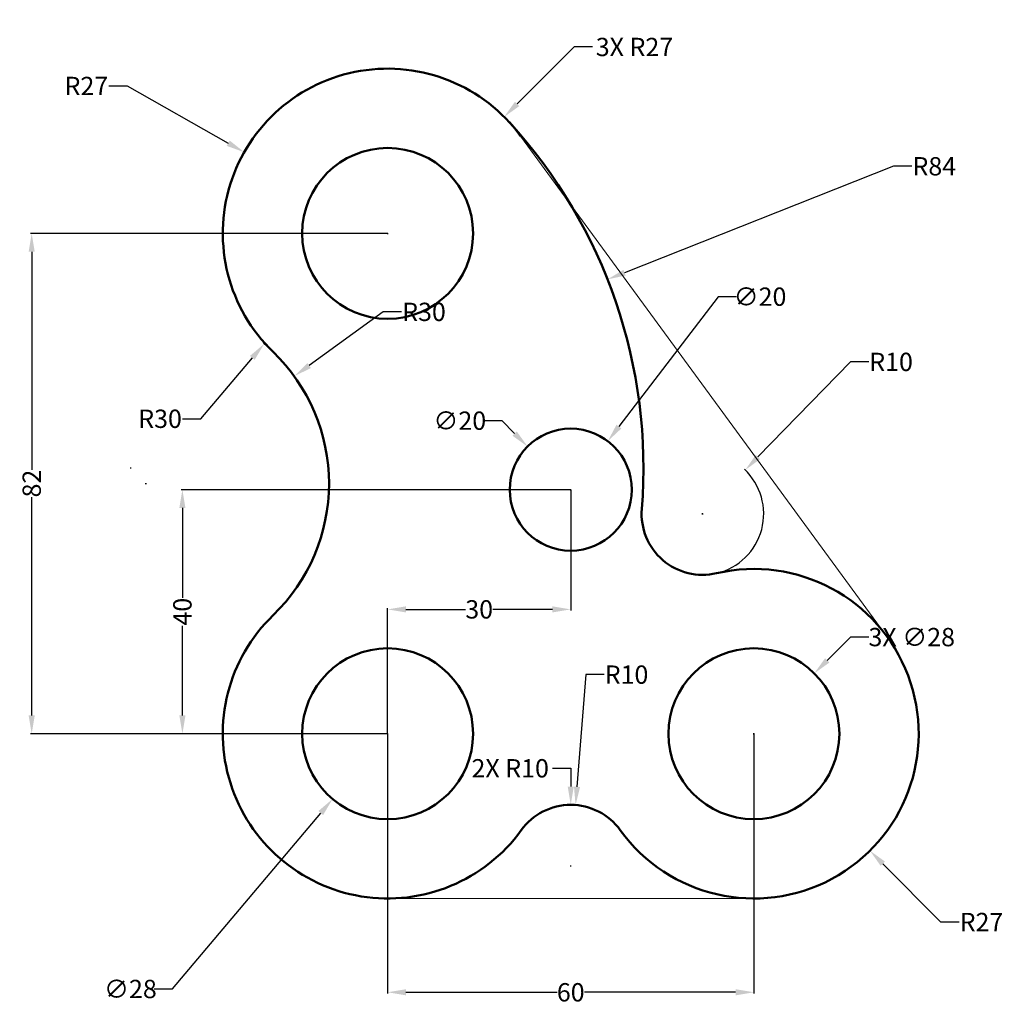
# Model space of a CAD drawing. Units: millimetres. Extents: x -41 to 120, y -25 to 136.
import ezdxf

# ---------------------------------------------------------------- set-up
doc = ezdxf.new("R2010")
doc.units = ezdxf.units.MM
doc.header["$MEASUREMENT"] = 0
for name, color, linetype, lineweight in [('M-CONS', 8, 'Continuous', 18), ('M-DIMS', 3, 'Continuous', 25), ('M-OUTL', 7, 'Continuous', 50)]:
    doc.layers.add(name, color=color, linetype=linetype, lineweight=lineweight)
doc.styles.get("Standard").update_dxf_attribs({"font": 'arial.ttf'})
doc.dimstyles.get("Standard").update_dxf_attribs({"dimtxt": 3, "dimasz": 3, "dimexe": 0.18, "dimexo": 0.0625, "dimgap": 0.09, "dimtad": 0, "dimtih": 1, "dimtoh": 1, "dimdec": 1, "dimdsep": 46, "dimtxsty": 'Standard', "dimcen": 0.09, "dimadec": 0, "dimazin": 0, "dimtfac": 1, "dimtdec": 1, "dimtofl": 0, "dimtmove": 0, "dimatfit": 3, "dimfxl": 1, "dimtolj": 1, "dimtzin": 0, "dimarcsym": 0})

# ---------------------------------------------------------------- blocks, each defined once
blk = doc.blocks.new('*D1')
at = {"layer": 'Defpoints', "color": 0, "transparency": 16777216}
for p in [(19.33, 18.94), (79.33, 18.94), (79.33, -23.43)]:
    blk.add_point(p, dxfattribs=at)
at = {"layer": 'M-DIMS', "color": 0, "lineweight": -2, "transparency": 16777216}
for p, q in [((19.33, 18.88), (19.33, -23.61)), ((79.33, 18.88), (79.33, -23.61)), ((22.33, -23.43), (47.09, -23.43)), ((76.33, -23.43), (51.57, -23.43))]:
    blk.add_line(p, q, dxfattribs=at)
at = {"layer": 'M-DIMS', "color": 0, "transparency": 16777216}
for points in [[(22.33, -22.93), (22.33, -23.93), (19.33, -23.43)], [(76.33, -22.93), (76.33, -23.93), (79.33, -23.43)]]:
    blk.add_solid(points, dxfattribs=at)
at = {"layer": 'M-DIMS', "color": 0, "transparency": 16777216, "insert": (49.33, -23.43), "char_height": 3, "attachment_point": 5}
blk.add_mtext('\\A1;60', dxfattribs=at)
blk = doc.blocks.new('*D2')
at = {"layer": 'Defpoints', "color": 0, "transparency": 16777216}
for p in [(-38.98, 100.94), (19.33, 100.94), (19.33, 18.94)]:
    blk.add_point(p, dxfattribs=at)
at = {"layer": 'M-DIMS', "color": 0, "lineweight": -2, "transparency": 16777216}
for p, q in [((19.27, 100.94), (-39.16, 100.94)), ((-38.98, 97.94), (-38.98, 62.17)), ((-38.98, 21.94), (-38.98, 57.72)), ((19.27, 18.94), (-39.16, 18.94))]:
    blk.add_line(p, q, dxfattribs=at)
at = {"layer": 'M-DIMS', "color": 0, "transparency": 16777216}
for points in [[(-39.48, 97.94), (-38.48, 97.94), (-38.98, 100.94)], [(-39.48, 21.94), (-38.48, 21.94), (-38.98, 18.94)]]:
    blk.add_solid(points, dxfattribs=at)
at = {"layer": 'M-DIMS', "color": 0, "transparency": 16777216, "insert": (-38.98, 59.94), "char_height": 3, "attachment_point": 5, "rotation": 90}
blk.add_mtext('\\A1;82', dxfattribs=at)
blk = doc.blocks.new('*D3')
at = {"layer": 'Defpoints', "color": 0, "transparency": 16777216}
for p in [(-14.29, 58.94), (49.33, 58.94), (19.33, 18.94)]:
    blk.add_point(p, dxfattribs=at)
at = {"layer": 'M-DIMS', "color": 0, "lineweight": -2, "transparency": 16777216}
for p, q in [((49.27, 58.94), (-14.47, 58.94)), ((-14.29, 55.94), (-14.29, 41.23)), ((-14.29, 21.94), (-14.29, 36.65)), ((19.27, 18.94), (-14.47, 18.94))]:
    blk.add_line(p, q, dxfattribs=at)
at = {"layer": 'M-DIMS', "color": 0, "transparency": 16777216}
for points in [[(-14.79, 55.94), (-13.79, 55.94), (-14.29, 58.94)], [(-14.79, 21.94), (-13.79, 21.94), (-14.29, 18.94)]]:
    blk.add_solid(points, dxfattribs=at)
at = {"layer": 'M-DIMS', "color": 0, "transparency": 16777216, "insert": (-14.29, 38.94), "char_height": 3, "attachment_point": 5, "rotation": 90}
blk.add_mtext('\\A1;40', dxfattribs=at)
blk = doc.blocks.new('*D4')
at = {"layer": 'Defpoints', "color": 0, "transparency": 16777216}
for p in [(49.33, 58.94), (49.33, 39.32), (19.33, 18.94)]:
    blk.add_point(p, dxfattribs=at)
at = {"layer": 'M-DIMS', "color": 0, "lineweight": -2, "transparency": 16777216}
for p, q in [((49.33, 58.88), (49.33, 39.14)), ((19.33, 19), (19.33, 39.5)), ((22.33, 39.32), (32.1, 39.32)), ((46.33, 39.32), (36.56, 39.32))]:
    blk.add_line(p, q, dxfattribs=at)
at = {"layer": 'M-DIMS', "color": 0, "transparency": 16777216}
for points in [[(22.33, 39.82), (22.33, 38.82), (19.33, 39.32)], [(46.33, 39.82), (46.33, 38.82), (49.33, 39.32)]]:
    blk.add_solid(points, dxfattribs=at)
at = {"layer": 'M-DIMS', "color": 0, "transparency": 16777216, "insert": (34.33, 39.32), "char_height": 3, "attachment_point": 5}
blk.add_mtext('\\A1;30', dxfattribs=at)
blk = doc.blocks.new('*D5')
at = {"layer": 'Defpoints', "color": 0, "transparency": 16777216}
for p in [(-0.89, 82.84), (-20.27, 59.94)]:
    blk.add_point(p, dxfattribs=at)
at = {"layer": 'M-DIMS', "color": 0, "lineweight": -2, "transparency": 16777216}
for p, q in [((-11.28, 70.56), (-2.82, 80.55)), ((-14.28, 70.56), (-11.28, 70.56))]:
    blk.add_line(p, q, dxfattribs=at)
blk.add_arc((-20.27, 59.94), 30, 46.1159, 50.1018, dxfattribs=at)
at = {"layer": 'M-DIMS', "color": 0, "transparency": 16777216}
blk.add_solid([(-3.21, 80.87), (-2.44, 80.23), (-0.89, 82.84)], dxfattribs=at)
at = {"layer": 'M-DIMS', "color": 0, "transparency": 16777216, "insert": (-17.95, 70.56), "char_height": 3, "attachment_point": 5}
blk.add_mtext('\\A1;R30', dxfattribs=at)
blk = doc.blocks.new('*D6')
at = {"layer": 'Defpoints', "color": 0, "transparency": 16777216}
for p in [(-4.16, 114.24), (19.33, 100.94)]:
    blk.add_point(p, dxfattribs=at)
at = {"layer": 'M-DIMS', "color": 0, "lineweight": -2, "transparency": 16777216}
for p, q in [((-26.34, 125.1), (-23.34, 125.1)), ((-23.34, 125.1), (-6.78, 115.72)), ((19.24, 100.94), (19.42, 100.94)), ((19.33, 100.85), (19.33, 101.03))]:
    blk.add_line(p, q, dxfattribs=at)
at = {"layer": 'M-DIMS', "color": 0, "transparency": 16777216}
blk.add_solid([(-6.53, 116.15), (-7.02, 115.28), (-4.16, 114.24)], dxfattribs=at)
at = {"layer": 'M-DIMS', "color": 0, "transparency": 16777216, "insert": (-30.02, 125.1), "char_height": 3, "attachment_point": 5}
blk.add_mtext('\\A1;R27', dxfattribs=at)
blk = doc.blocks.new('*D7')
at = {"layer": 'Defpoints', "color": 0, "transparency": 16777216}
for p in [(28.36, 29.64), (10.31, 8.24)]:
    blk.add_point(p, dxfattribs=at)
at = {"layer": 'M-DIMS', "color": 0, "lineweight": -2, "transparency": 16777216}
for p, q in [((19.24, 18.94), (19.42, 18.94)), ((19.33, 18.85), (19.33, 19.03)), ((-15.94, -22.89), (8.37, 5.94)), ((-18.94, -22.89), (-15.94, -22.89))]:
    blk.add_line(p, q, dxfattribs=at)
at = {"layer": 'M-DIMS', "color": 0, "transparency": 16777216}
blk.add_solid([(7.99, 6.27), (8.76, 5.62), (10.31, 8.24)], dxfattribs=at)
at = {"layer": 'M-DIMS', "color": 0, "transparency": 16777216, "insert": (-22.81, -22.89), "char_height": 3, "attachment_point": 5}
blk.add_mtext('\\A1;∅28', dxfattribs=at)
blk = doc.blocks.new('*D8')
at = {"layer": 'Defpoints', "color": 0, "transparency": 16777216}
for p in [(50.12, 7.25), (49.33, -2.72)]:
    blk.add_point(p, dxfattribs=at)
at = {"layer": 'M-DIMS', "color": 0, "lineweight": -2, "transparency": 16777216}
for p, q in [((51.8, 28.63), (50.35, 10.24)), ((54.8, 28.63), (51.8, 28.63)), ((49.24, -2.72), (49.42, -2.72)), ((49.33, -2.81), (49.33, -2.63))]:
    blk.add_line(p, q, dxfattribs=at)
at = {"layer": 'M-DIMS', "color": 0, "transparency": 16777216}
blk.add_solid([(49.86, 10.28), (50.85, 10.2), (50.12, 7.25)], dxfattribs=at)
at = {"layer": 'M-DIMS', "color": 0, "transparency": 16777216, "insert": (58.47, 28.63), "char_height": 3, "attachment_point": 5}
blk.add_mtext('\\A1;R10', dxfattribs=at)
blk = doc.blocks.new('*D9')
at = {"layer": 'Defpoints', "color": 0, "transparency": 16777216}
for p in [(55.4, 66.89), (43.27, 50.99)]:
    blk.add_point(p, dxfattribs=at)
at = {"layer": 'M-DIMS', "color": 0, "lineweight": -2, "transparency": 16777216}
for p, q in [((73.47, 90.57), (57.22, 69.27)), ((76.47, 90.57), (73.47, 90.57)), ((49.24, 58.94), (49.42, 58.94)), ((49.33, 58.85), (49.33, 59.03))]:
    blk.add_line(p, q, dxfattribs=at)
at = {"layer": 'M-DIMS', "color": 0, "transparency": 16777216}
blk.add_solid([(56.82, 69.58), (57.62, 68.97), (55.4, 66.89)], dxfattribs=at)
at = {"layer": 'M-DIMS', "color": 0, "transparency": 16777216, "insert": (80.34, 90.57), "char_height": 3, "attachment_point": 5}
blk.add_mtext('\\A1;∅20', dxfattribs=at)
blk = doc.blocks.new('*D10')
at = {"layer": 'Defpoints', "color": 0, "transparency": 16777216}
for p in [(77.91, 62.15), (70.94, 54.98)]:
    blk.add_point(p, dxfattribs=at)
at = {"layer": 'M-DIMS', "color": 0, "lineweight": -2, "transparency": 16777216}
for p, q in [((95.14, 79.88), (80, 64.3)), ((98.14, 79.88), (95.14, 79.88)), ((70.85, 54.98), (71.03, 54.98)), ((70.94, 54.89), (70.94, 55.07))]:
    blk.add_line(p, q, dxfattribs=at)
blk.add_arc((70.94, 54.98), 10, 283.4727, 46.8536, dxfattribs=at)
at = {"layer": 'M-DIMS', "color": 0, "transparency": 16777216}
blk.add_solid([(79.64, 64.65), (80.35, 63.95), (77.91, 62.15)], dxfattribs=at)
at = {"layer": 'M-DIMS', "color": 0, "transparency": 16777216, "insert": (101.81, 79.88), "char_height": 3, "attachment_point": 5}
blk.add_mtext('\\A1;R10', dxfattribs=at)
blk = doc.blocks.new('*D11')
at = {"layer": 'Defpoints', "color": 0, "transparency": 16777216}
for p in [(79.33, 18.94), (98.35, -0.23)]:
    blk.add_point(p, dxfattribs=at)
at = {"layer": 'M-DIMS', "color": 0, "lineweight": -2, "transparency": 16777216}
for p, q in [((79.24, 18.94), (79.42, 18.94)), ((79.33, 18.85), (79.33, 19.03)), ((109.95, -11.92), (100.46, -2.36)), ((112.95, -11.92), (109.95, -11.92))]:
    blk.add_line(p, q, dxfattribs=at)
at = {"layer": 'M-DIMS', "color": 0, "transparency": 16777216}
blk.add_solid([(100.81, -2.01), (100.1, -2.71), (98.35, -0.23)], dxfattribs=at)
at = {"layer": 'M-DIMS', "color": 0, "transparency": 16777216, "insert": (116.62, -11.92), "char_height": 3, "attachment_point": 5}
blk.add_mtext('\\A1;R27', dxfattribs=at)
blk = doc.blocks.new('HOLE-D28')
blk.add_circle((14, 14), 14)
blk = doc.blocks.new('*D13')
at = {"layer": 'Defpoints', "color": 0, "transparency": 16777216}
for p in [(89.23, 28.84), (69.43, 9.04)]:
    blk.add_point(p, dxfattribs=at)
at = {"layer": 'M-DIMS', "color": 0, "lineweight": -2, "transparency": 16777216}
for p, q in [((95.17, 34.78), (91.35, 30.96)), ((98.17, 34.78), (95.17, 34.78)), ((79.24, 18.94), (79.42, 18.94)), ((79.33, 18.85), (79.33, 19.03))]:
    blk.add_line(p, q, dxfattribs=at)
at = {"layer": 'M-DIMS', "color": 0, "transparency": 16777216}
blk.add_solid([(91, 31.32), (91.71, 30.61), (89.23, 28.84)], dxfattribs=at)
at = {"layer": 'M-DIMS', "color": 0, "transparency": 16777216, "insert": (105.19, 34.78), "char_height": 3, "attachment_point": 5}
blk.add_mtext('\\A1;3X ∅28', dxfattribs=at)
blk = doc.blocks.new('*D14')
at = {"layer": 'Defpoints', "color": 0, "transparency": 16777216}
for p in [(42.26, 66.01), (56.4, 51.87)]:
    blk.add_point(p, dxfattribs=at)
at = {"layer": 'M-DIMS', "color": 0, "lineweight": -2, "transparency": 16777216}
for p, q in [((35.02, 70.25), (38.02, 70.25)), ((38.02, 70.25), (40.14, 68.13)), ((49.24, 58.94), (49.42, 58.94)), ((49.33, 58.85), (49.33, 59.03))]:
    blk.add_line(p, q, dxfattribs=at)
at = {"layer": 'M-DIMS', "color": 0, "transparency": 16777216}
blk.add_solid([(40.49, 68.48), (39.78, 67.78), (42.26, 66.01)], dxfattribs=at)
at = {"layer": 'M-DIMS', "color": 0, "transparency": 16777216, "insert": (31.15, 70.25), "char_height": 3, "attachment_point": 5}
blk.add_mtext('\\A1;∅20', dxfattribs=at)
blk = doc.blocks.new('*D15')
at = {"layer": 'Defpoints', "color": 0, "transparency": 16777216}
for p in [(38.42, 120.03), (19.33, 100.94)]:
    blk.add_point(p, dxfattribs=at)
at = {"layer": 'M-DIMS', "color": 0, "lineweight": -2, "transparency": 16777216}
for p, q in [((49.88, 131.49), (40.54, 122.15)), ((52.88, 131.49), (49.88, 131.49)), ((19.24, 100.94), (19.42, 100.94)), ((19.33, 100.85), (19.33, 101.03))]:
    blk.add_line(p, q, dxfattribs=at)
at = {"layer": 'M-DIMS', "color": 0, "transparency": 16777216}
blk.add_solid([(40.19, 122.51), (40.9, 121.8), (38.42, 120.03)], dxfattribs=at)
at = {"layer": 'M-DIMS', "color": 0, "transparency": 16777216, "insert": (59.77, 131.49), "char_height": 3, "attachment_point": 5}
blk.add_mtext('\\A1;3X R27', dxfattribs=at)
blk = doc.blocks.new('*D16')
at = {"layer": 'Defpoints', "color": 0, "transparency": 16777216}
for p in [(49.33, 7.28), (49.33, -2.72)]:
    blk.add_point(p, dxfattribs=at)
at = {"layer": 'M-DIMS', "color": 0, "lineweight": -2, "transparency": 16777216}
for p, q in [((46.33, 13.28), (49.33, 13.28)), ((49.33, 13.28), (49.33, 10.28)), ((49.24, -2.72), (49.42, -2.72)), ((49.33, -2.81), (49.33, -2.63))]:
    blk.add_line(p, q, dxfattribs=at)
at = {"layer": 'M-DIMS', "color": 0, "transparency": 16777216}
blk.add_solid([(49.83, 10.28), (48.83, 10.28), (49.33, 7.28)], dxfattribs=at)
at = {"layer": 'M-DIMS', "color": 0, "transparency": 16777216, "insert": (39.41, 13.28), "char_height": 3, "attachment_point": 5}
blk.add_mtext('\\A1;2X R10', dxfattribs=at)
blk = doc.blocks.new('*D17')
at = {"layer": 'Defpoints', "color": 0, "transparency": 16777216}
for p in [(4.04, 77.53), (-20.27, 59.94)]:
    blk.add_point(p, dxfattribs=at)
at = {"layer": 'M-DIMS', "color": 0, "lineweight": -2, "transparency": 16777216}
for p, q in [((18.62, 88.08), (6.47, 79.29)), ((21.62, 88.08), (18.62, 88.08)), ((-20.36, 59.94), (-20.18, 59.94)), ((-20.27, 59.85), (-20.27, 60.03))]:
    blk.add_line(p, q, dxfattribs=at)
at = {"layer": 'M-DIMS', "color": 0, "transparency": 16777216}
blk.add_solid([(6.18, 79.69), (6.76, 78.88), (4.04, 77.53)], dxfattribs=at)
at = {"layer": 'M-DIMS', "color": 0, "transparency": 16777216, "insert": (25.29, 88.08), "char_height": 3, "attachment_point": 5}
blk.add_mtext('\\A1;R30', dxfattribs=at)
blk = doc.blocks.new('*D18')
at = {"layer": 'Defpoints', "color": 0, "transparency": 16777216}
for p in [(55.35, 93.4), (-22.76, 62.51)]:
    blk.add_point(p, dxfattribs=at)
at = {"layer": 'M-DIMS', "color": 0, "lineweight": -2, "transparency": 16777216}
for p, q in [((102.22, 111.94), (58.14, 94.5)), ((105.22, 111.94), (102.22, 111.94)), ((-22.85, 62.51), (-22.67, 62.51)), ((-22.76, 62.42), (-22.76, 62.6))]:
    blk.add_line(p, q, dxfattribs=at)
at = {"layer": 'M-DIMS', "color": 0, "transparency": 16777216}
blk.add_solid([(57.96, 94.97), (58.33, 94.04), (55.35, 93.4)], dxfattribs=at)
at = {"layer": 'M-DIMS', "color": 0, "transparency": 16777216, "insert": (108.89, 111.94), "char_height": 3, "attachment_point": 5}
blk.add_mtext('\\A1;R84', dxfattribs=at)

msp = doc.modelspace()

# ---------------------------------------------------------------- linework, layer by layer
at = {"layer": 'M-CONS'}
for p, q in [((101.12, 34.88), (41.12, 116.88)), ((19.33, -8.06), (79.33, -8.06))]:
    msp.add_line(p, q, dxfattribs=at)
msp.add_arc((-22.76, 62.51), 84, 302.8523, 303.2091, dxfattribs=at)
at = {"layer": 'M-OUTL'}
msp.add_circle((49.33, 58.94), 10, dxfattribs=at)
for centre, radius, start, end in [((19.33, 100.94), 27, 36.1932, 225.9966), ((-22.76, 62.51), 84, 355.4047, 42.3983), ((-20.27, 59.94), 30, 314.0034, 45.9966), ((70.94, 54.98), 10, 175.4047, 283.1146), ((79.33, 18.94), 27, 215.8248, 103.1146), ((19.33, 18.94), 27, 134.0034, 324.1752), ((49.33, -2.72), 10, 35.8248, 144.1752)]:
    msp.add_arc(centre, radius, start, end, dxfattribs=at)

# ---------------------------------------------------------------- block references
for p in [(5.33, 86.94), (5.33, 4.94), (65.33, 4.94)]:
    msp.add_blockref('HOLE-D28', p, dxfattribs=at)

# ---------------------------------------------------------------- dimensions: what is measured, and where the dimension line sits
at = {"layer": 'M-DIMS'}
dim = msp.add_radius_dim(center=(19.33, 100.94), mpoint=(38.42, 120.03), text='3X <>', dimstyle='Standard', override={"dimdec": 0, "dimlfac": 1, "dimrnd": 0, "dimzin": 0, "dimdsep": 46, "dimlunit": 2}, dxfattribs=at)
dim.commit()
dim.dimension.update_dxf_attribs({"geometry": '*D15', "text_midpoint": (59.77, 131.49), "dimtype": 164})
at = {"layer": 'M-DIMS', "transparency": 33554610}
for center, mpoint, picture, middle in [((19.33, 100.94), (-4.16, 114.24), '*D6', (-30.02, 125.1)), ((-20.27, 59.94), (-0.89, 82.84), '*D5', (-17.95, 70.56)), ((70.94, 54.98), (77.91, 62.15), '*D10', (101.81, 79.88)), ((49.33, -2.72), (50.12, 7.25), '*D8', (58.47, 28.63)), ((79.33, 18.94), (98.35, -0.23), '*D11', (116.62, -11.92))]:
    dim = msp.add_radius_dim(center=center, mpoint=mpoint, dimstyle='Standard', override={"dimclrd": 0, "dimclre": 0, "dimclrt": 0}, dxfattribs=at)
    dim.commit()
    dim.dimension.update_dxf_attribs({"geometry": picture, "text_midpoint": middle, "dimtype": 164})
at = {"layer": 'M-DIMS'}
for center, mpoint, picture, middle in [((-22.76, 62.51), (55.35, 93.4), '*D18', (108.89, 111.94)), ((-20.27, 59.94), (4.04, 77.53), '*D17', (25.29, 88.08))]:
    dim = msp.add_radius_dim(center=center, mpoint=mpoint, dimstyle='Standard', override={"dimdec": 0, "dimlfac": 1, "dimrnd": 0, "dimzin": 0, "dimdsep": 46, "dimlunit": 2}, dxfattribs=at)
    dim.commit()
    dim.dimension.update_dxf_attribs({"geometry": picture, "text_midpoint": middle, "dimtype": 164})
at = {"layer": 'M-DIMS', "transparency": 33554610}
for base, p2, picture, middle in [((-38.98, 100.94), (19.33, 100.94), '*D2', (-38.98, 59.94)), ((-14.29, 58.94), (49.33, 58.94), '*D3', (-14.29, 38.94))]:
    dim = msp.add_linear_dim(base=base, p1=(19.33, 18.94), p2=p2, angle=90, dimstyle='Standard', override={"dimclrd": 0, "dimclre": 0, "dimclrt": 0}, dxfattribs=at)
    dim.commit()
    dim.dimension.update_dxf_attribs({"geometry": picture, "text_midpoint": middle, "text_rotation": 90})
for p1, p2, picture, middle in [((43.27, 50.99), (55.4, 66.89), '*D9', (80.34, 90.57)), ((28.36, 29.64), (10.31, 8.24), '*D7', (-22.81, -22.89))]:
    dim = msp.add_diameter_dim_2p(p1=p1, p2=p2, dimstyle='Standard', override={"dimclrd": 0, "dimclre": 0, "dimclrt": 0}, dxfattribs=at)
    dim.commit()
    dim.dimension.update_dxf_attribs({"geometry": picture, "text_midpoint": middle, "dimtype": 163})
at = {"layer": 'M-DIMS'}
dim = msp.add_diameter_dim_2p(p1=(56.4, 51.87), p2=(42.26, 66.01), dimstyle='Standard', override={"dimdec": 0, "dimlfac": 1, "dimrnd": 0, "dimzin": 0, "dimdsep": 46, "dimlunit": 2}, dxfattribs=at)
dim.commit()
dim.dimension.update_dxf_attribs({"geometry": '*D14', "text_midpoint": (31.15, 70.25), "dimtype": 163})
at = {"layer": 'M-DIMS', "transparency": 33554610}
for base, p2, picture, middle in [((49.33, 39.32), (49.33, 58.94), '*D4', (34.33, 39.32)), ((79.33, -23.43), (79.33, 18.94), '*D1', (49.33, -23.43))]:
    dim = msp.add_linear_dim(base=base, p1=(19.33, 18.94), p2=p2, dimstyle='Standard', override={"dimclrd": 0, "dimclre": 0, "dimclrt": 0}, dxfattribs=at)
    dim.commit()
    dim.dimension.update_dxf_attribs({"geometry": picture, "text_midpoint": middle})
at = {"layer": 'M-DIMS'}
dim = msp.add_diameter_dim_2p(p1=(69.43, 9.04), p2=(89.23, 28.84), text='3X <>', dimstyle='Standard', override={"dimdec": 0, "dimlfac": 1, "dimrnd": 0, "dimzin": 0, "dimdsep": 46, "dimlunit": 2}, dxfattribs=at)
dim.commit()
dim.dimension.update_dxf_attribs({"geometry": '*D13', "text_midpoint": (105.19, 34.78), "dimtype": 163})
dim = msp.add_radius_dim(center=(49.33, -2.72), mpoint=(49.33, 7.28), text='2X <>', dimstyle='Standard', override={"dimdec": 0, "dimlfac": 1, "dimrnd": 0, "dimzin": 0, "dimdsep": 46, "dimlunit": 2}, dxfattribs=at)
dim.commit()
dim.dimension.update_dxf_attribs({"geometry": '*D16', "text_midpoint": (39.41, 13.28)})

doc.saveas('drawing.dxf')
